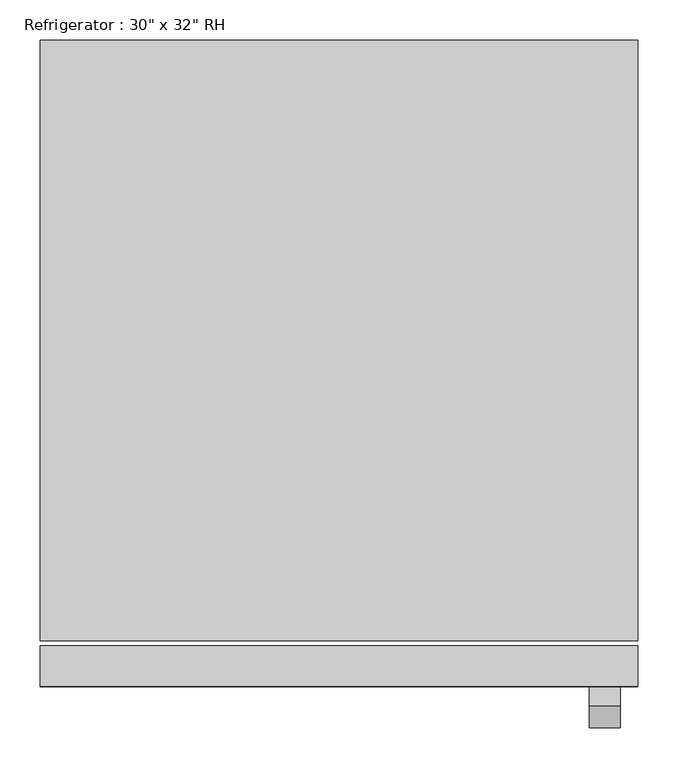
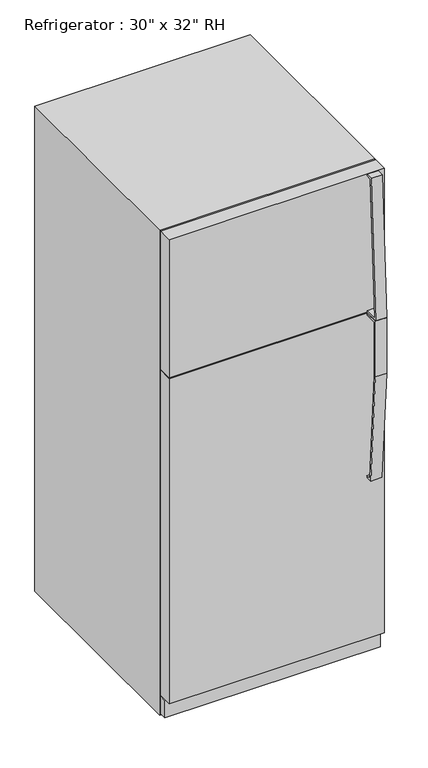
"""IFC4 building model written with IfcOpenShell, lengths in millimetres: proxy geometry."""

from ifc_helpers import new_model, si_unit, frame, origin, origin_with_axes, place, context, project, spatial, polyline, outline, extrude, source, transform, mapped, element, save


def proxy_a13a33b2(model_context):
    return source(origin(), model_context, "Body", "SweptSolid", [
        extrude(outline(polyline([(-417.9010285, 1262.0625), (-462.3510285, 1262.0625), (-462.3510285, 1065.4342469), (-434.8723987, 672.4715334), (-417.9010285, 672.4715334), (-417.9010285, 666.1370017), (-440.7949512, 666.1370017), (-468.7010285, 1065.2125), (-468.7010285, 1268.4125), (-417.9010285, 1268.4125), (-417.9010285, 1262.0625)])), frame((312.7375, 0.0, 0.0), z_axis=(1.0, 0.0, 0.0), x_axis=(0.0, 1.0, 0.0)), (0.0, 0.0, 1.0), 38.4332978),
        extrude(outline(polyline([(-442.739413, 1778.0), (-418.6780855, 1778.0), (-418.6780855, 1771.65), (-437.5263449, 1771.65), (-463.4007207, 1277.9375), (-418.6780855, 1277.9375), (-418.6780855, 1271.5875), (-469.2793675, 1271.5875), (-442.739413, 1778.0)])), frame((312.7375, 0.0, 0.0), z_axis=(1.0, 0.0, 0.0), x_axis=(0.0, 1.0, 0.0)), (0.0, 0.0, 1.0), 38.4332978),
        extrude(outline(polyline([(373.0625, -367.1010285), (373.0625, -392.5010285), (-373.0625, -392.5010285), (-373.0625, -367.1010285), (373.0625, -367.1010285)])), frame((0.0, 0.0, 9.3816357), z_axis=(0.0, 0.0, 1.0), x_axis=(1.0, 0.0, 0.0)), (0.0, 0.0, 1.0), 63.5),
        extrude(outline(polyline([(373.0625, -367.1010285), (373.0625, -417.9010285), (-373.0625, -417.9010285), (-373.0625, -367.1010285), (373.0625, -367.1010285)])), frame((0.0, 0.0, 76.2), z_axis=(0.0, 0.0, 1.0), x_axis=(1.0, 0.0, 0.0)), (0.0, 0.0, 1.0), 1192.2125),
        extrude(outline(polyline([(373.0625, -367.1010285), (373.0625, -417.9010285), (-373.0625, -417.9010285), (-373.0625, -367.1010285), (373.0625, -367.1010285)])), frame((0.0, 0.0, 1271.5875), z_axis=(0.0, 0.0, 1.0), x_axis=(1.0, 0.0, 0.0)), (0.0, 0.0, 1.0), 506.4125),
        extrude(outline(polyline([(373.0625, 388.5489715), (373.0625, -360.7510285), (-373.0625, -360.7510285), (-373.0625, 388.5489715), (373.0625, 388.5489715)])), origin_with_axes(), (0.0, 0.0, 1.0), 1778.0),
    ])


if __name__ == "__main__":
    model = new_model("IFC4")
    model_context = context("Model", 3, world=origin())
    ifc_project = project(units=[si_unit("LENGTHUNIT", "METRE", prefix="MILLI")], contexts=[model_context])
    site = spatial("IfcSite", under=ifc_project)
    building = spatial("IfcBuilding", under=site)
    placement = place(None, origin())
    proxy_shape = proxy_a13a33b2(model_context)
    element("IfcBuildingElementProxy", 1, Name="Refrigerator : 30\" x 32\" RH", ObjectType="Refrigerator : 30\" x 32\" RH", at=placement, inside=building, context=model_context, shape_type="MappedRepresentation", body=[
        mapped(proxy_shape, transform((0.0, 0.0, 0.0), x_axis=(1.0, 0.0, 0.0), y_axis=(0.0, 1.0, 0.0), z_axis=(0.0, 0.0, 1.0))),
    ])
    save(model, "model.ifc")

# Revit data of these elements
# Type "Refrigerator : 30\" x 32\" RH"
#   Label = "REF."
#   Assembly Code = "E1090400"
#   Depth = 2' - 7 3/4"
#   Handle = 2' - 3"
#   Height = 5' - 10"
#   Rear Clearance = 0' - 2"
#   Top Door Height = 1' - 8"
#   Width = 2' - 5 3/8"
#   Material = Steel, Paint Finish, Ivory, Glossy
#   Default Elevation = 0
# Element 1 (IfcBuildingElementProxy, "Refrigerator : 30\" x 32\" RH")
#   Materials on its faces: "Steel, Paint Finish, Ivory, Glossy", "Steel, Chrome Plated"
# Materials
#   "Steel, Paint Finish, Ivory, Glossy": class "Metal", colour RGB 247 247 239, transparency 0, Description = "Steel, paint finish, ivory, glossy", Cost = 0
#   "Steel, Chrome Plated": class "Metal", colour RGB 17 17 17, transparency 0, Description = "Chromiuim plated steel", Cost = 0
